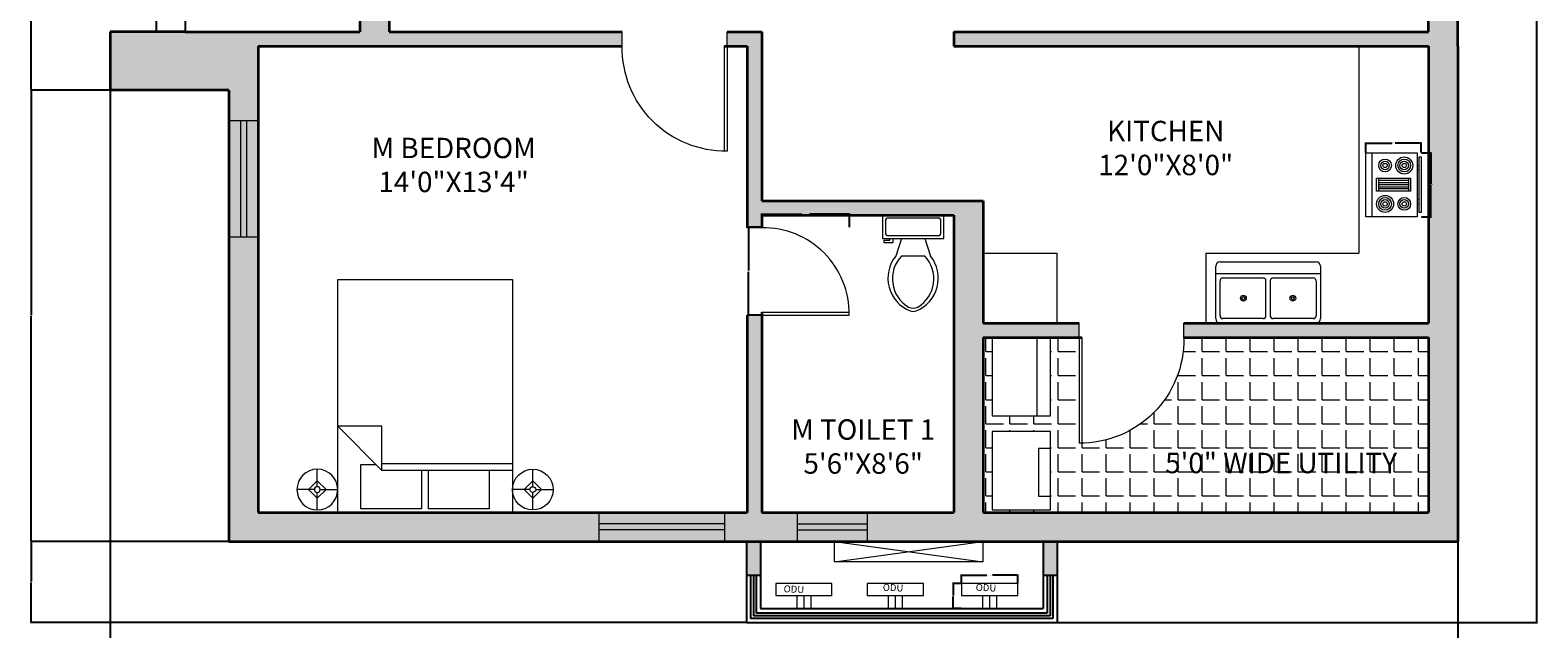
# Model space of a CAD drawing. Units: inches. Extents: x -382 to 250, y 518 to 1732.
# Tile 5 of 8: x -270 to 247, y 1167 to 1373. Entities that reach past the tile are written whole.
import ezdxf

# ---------------------------------------------------------------- set-up
doc = ezdxf.new("R2010")
doc.units = ezdxf.units.IN
doc.header["$MEASUREMENT"] = 0
for name, color, linetype, lineweight in [('A-ANNO-DIMS', 2, 'Continuous', 18), ('A-AREA-IDEN', 7, 'Continuous', 18), ('A-DOOR', 3, 'Continuous', 18), ('A-EQPM', 9, 'Continuous', 18), ('A-FLOR-CASE', 8, 'Continuous', 18), ('A-FLOR-EDGE', 7, 'Continuous', 25), ('A-FLOR-FIXT', 8, 'Continuous', 18), ('A-FLOR-PATT', 9, 'Continuous', 13), ('A-FLOR-SHFT', 8, 'Continuous', 18), ('A-FURN', 8, 'Continuous', 18), ('A-GLAZ', 4, 'Continuous', 18), ('A-WALL', 7, 'Continuous', 35), ('M-ANNO-TEXT', 7, 'Continuous', 13), ('M-HVAC-EQPM', 4, 'Continuous', 18)]:
    doc.layers.add(name, color=color, linetype=linetype, lineweight=lineweight)
doc.layers.add('A-GLAZ-PATT', color=143, linetype='Continuous', lineweight=13, true_color=0x7aafdf)
doc.layers.add('A-WALL-PATT', color=251, linetype='Continuous', lineweight=13, true_color=0x636466)
doc.styles.get("Standard").update_dxf_attribs({"font": 'arial.ttf'})
doc.dimstyles.get("Standard").update_dxf_attribs({"dimtxt": 0.18, "dimasz": 0.18, "dimexe": 0.18, "dimexo": 0.0625, "dimgap": 0.09, "dimtad": 0, "dimtih": 1, "dimtoh": 1, "dimdec": 4, "dimzin": 0, "dimdsep": 46, "dimtxsty": 'Standard', "dimcen": 0.09, "dimadec": 0, "dimazin": 0, "dimtfac": 1, "dimtdec": 4, "dimtofl": 0, "dimtmove": 0, "dimatfit": 3, "dimfxl": 1, "dimtolj": 1, "dimtzin": 0, "dimarcsym": 0})

# ---------------------------------------------------------------- blocks, each defined once
blk = doc.blocks.new('Bed - Queen')
for p, q in [((0, -80.00003), (0, 0)), ((0, 0), (59.99999, 0)), ((59.99999, 0), (59.99999, -80.00003)), ((7.99999, -1.2), (28.79998, -1.2)), ((7.99999, -14.4), (7.99999, -1.2)), ((28.79998, -1.2), (28.79998, -14.4)), ((31.19999, -1.2), (51.99999, -1.2)), ((31.19999, -14.4), (31.19999, -1.2)), ((51.99999, -1.2), (51.99999, -16.4)), ((0, -14.4), (44.8, -14.4)), ((59.99999, -29.6), (44.8, -14.4)), ((44.8, -14.4), (44.8, -29.6)), ((44.8, -16.8), (0, -16.8)), ((51.99999, -16.4), (46.79936, -16.4)), ((44.8, -29.6), (59.99999, -29.6)), ((59.99999, -80.00003), (0, -80.00003))]:
    blk.add_line(p, q)
blk = doc.blocks.new('Lamp - Table')
for p, q in [((0, 7), (0, 1)), ((-1, 0), (-7, 0)), ((0, 3), (-3, 0)), ((-3, 0), (0, -3)), ((3, 0), (0, 3)), ((0, -3), (3, 0)), ((1, 0), (7, 0)), ((0, -1), (0, -7))]:
    blk.add_line(p, q)
for radius in [7, 1]:
    blk.add_circle((0, 0), radius)
blk = doc.blocks.new('Range-Oven - 30 in top')
for p, q in [((0, -3), (30, -3)), ((12, -6), (18, -6)), ((13, -20), (13, -6)), ((14, -6), (14, -20)), ((15, -20), (15, -6)), ((16, -6), (16, -20)), ((17, -20), (17, -6)), ((18, -20), (12, -20)), ((6, -24), (6, -25)), ((8, -25), (8, -24)), ((22, -25), (22, -24)), ((24, -24), (24, -25))]:
    blk.add_line(p, q)
for points in [[(0, -24), (0, 0), (30, 0), (30, -24)], [(12, -21), (12, -5), (18, -5), (18, -21)], [(2, -26), (2, -25), (28, -25), (28, -26)]]:
    blk.add_lwpolyline(points, close=True)
for centre, radius in [((6, -9), 4), ((6, -9), 3), ((6, -9), 2), ((24, -9), 3), ((24, -9), 2), ((6, -9), 1), ((24, -18), 4), ((24, -9), 1), ((6, -18), 3), ((6, -18), 2), ((6, -18), 1), ((24, -18), 3), ((24, -18), 2), ((24, -18), 1)]:
    blk.add_circle(centre, radius)
blk = doc.blocks.new('Sink-double - 36 in top')
for p, q in [((-18, -4), (18, -4)), ((-0.75, -18.5), (-0.75, -6.5)), ((0.75, -6.5), (0.75, -18.5))]:
    blk.add_line(p, q)
for points in [[(-16.5, 0), (16.5, 0)], [(-18, -19.5), (-18, -1.5)], [(18, -1.5), (18, -19.5)], [(-16.5, -18.5), (-16.5, -6.5)], [(-15.5, -5.5), (-1.75, -5.5)], [(1.75, -5.5), (15.5, -5.5)], [(16.5, -6.5), (16.5, -18.5)], [(-1.75, -19.5), (-15.5, -19.5)], [(15.5, -19.5), (1.75, -19.5)], [(16.5, -21), (-16.5, -21)]]:
    blk.add_lwpolyline(points)
for centre, radius in [((-8.5, -12.5), 1), ((-8.5, -12.5), 0.5), ((8.5, -12.5), 1), ((8.5, -12.5), 0.5)]:
    blk.add_circle(centre, radius)
for centre, radius, start, end in [((-16.5, -1.5), 1.5, 90, 180), ((16.5, -1.5), 1.5, 0, 90), ((-15.5, -6.5), 1, 90, 180), ((-1.75, -6.5), 1, 0, 90), ((1.75, -6.5), 1, 90, 180), ((15.5, -6.5), 1, 0, 90), ((-16.5, -19.5), 1.5, 180, 270), ((-15.5, -18.5), 1, 180, 270), ((-1.75, -18.5), 1, 270, 0), ((1.75, -18.5), 1, 180, 270), ((15.5, -18.5), 1, 270, 0), ((16.5, -19.5), 1.5, 270, 0)]:
    blk.add_arc(centre, radius, start, end)
blk = doc.blocks.new('Toilet - top')
for p, q in [((9.5, -6), (9.5, -2)), ((-10, -8.5), (-8, -8.5)), ((-10, -9.5), (-10, -8.5)), ((-7, -9.5), (-10, -9.5)), ((-8, -8.5), (-8, -8)), ((-7, -8), (-7, -9.5)), ((-4, -8), (-6, -14)), ((4, -8), (6, -14)), ((4, -14), (-4, -14))]:
    blk.add_line(p, q)
blk.add_lwpolyline([(10.5, -8), (10.5, 0), (-10.5, 0), (-10.5, -8)], close=True)
for points in [[(-9.5, -2), (-9.5, -6)], [(8.5, -1), (-8.5, -1)], [(-8.5, -7), (8.5, -7)]]:
    blk.add_lwpolyline(points)
for centre, radius, start, end in [((-8.62, -1.88), 0.884, 81.8699, 188.1301), ((8.62, -1.88), 0.884, 351.8699, 98.1301), ((-8.62, -6.12), 0.884, 171.8699, 278.1301), ((8.62, -6.12), 0.884, 261.8699, 8.1301), ((3.52, -21.58), 12.17, 141.4691, 247.9714), ((4.2, -21.82), 11.33, 136.3677, 238.9468), ((-3.52, -21.58), 12.17, 292.0284, 38.5307), ((-4.2, -21.82), 11.33, 301.053, 43.6321), ((0, -27.88), 4, 245.7318, 294.2682), ((0, -29), 4, 254.8605, 285.1395)]:
    blk.add_arc(centre, radius, start, end)
blk = doc.blocks.new('WIN-43_2IN')
for p, q in [((0, 10), (0, 0)), ((0, 6), (43.2, 6)), ((43.2, 10), (43.2, 0)), ((0, 4), (43.2, 4))]:
    blk.add_line(p, q)
blk = doc.blocks.new('WIN-40IN')
for p, q in [((10, 40), (0, 40)), ((4, 40), (4, 0)), ((6, 40), (6, 0)), ((10, 0), (0, 0))]:
    blk.add_line(p, q)
blk = doc.blocks.new('WIN-24IN')
for p, q in [((0, 0), (0, 10)), ((0, 6), (24, 6)), ((24, 0), (24, 10)), ((0, 4), (24, 4))]:
    blk.add_line(p, q)
blk = doc.blocks.new('DOOR-SWING-36IN')
for p, q in [((-1, 0), (-1, 36)), ((0, 0), (0, 36))]:
    blk.add_line(p, q)
blk.add_arc((-0.5, 0.5), 35.5, 89.1931, 180.8069)
blk = doc.blocks.new('DOOR-SWING-30IN')
for p, q in [((0, 1), (30, 1)), ((0, 0), (30, 0))]:
    blk.add_line(p, q)
blk.add_arc((0.5, 0.5), 29.5, 359.029, 90.971)
blk = doc.blocks.new('ODU-LEDGE-SMALL')
for p, q in [((7.26, 4.51), (7.26, 0)), ((9.66, 4.51), (9.66, 0)), ((12.06, 4.51), (12.06, 0))]:
    blk.add_line(p, q)
blk.add_lwpolyline([(0, 4.51), (19.32, 4.51), (19.32, 8.62), (0, 8.62)], close=True)
blk = doc.blocks.new('DOOR-SWING-36IN-OFFSET')
for p, q in [((0, 0), (0, 36)), ((1, -0.22), (1, 36))]:
    blk.add_line(p, q)
blk.add_arc((0.5, 0.5), 35.5, 359.1931, 90.8069)
blk = doc.blocks.new('*D48')
at = {"layer": 'A-ANNO-DIMS', "color": 0, "lineweight": -2, "transparency": 16777216}
for p, q in [((207.33, 1330.55), (210.75, 1330.55)), ((210.57, 1330.37), (210.57, 1319.75)), ((210.57, 1308.76), (210.57, 1319.38)), ((207.33, 1308.58), (210.75, 1308.58))]:
    blk.add_line(p, q, dxfattribs=at)
at = {"layer": 'A-ANNO-DIMS', "color": 0, "transparency": 16777216}
for points in [[(210.54, 1330.37), (210.6, 1330.37), (210.57, 1330.55)], [(210.54, 1308.76), (210.6, 1308.76), (210.57, 1308.58)]]:
    blk.add_solid(points, dxfattribs=at)
at = {"layer": 'Defpoints', "color": 0, "transparency": 16777216}
for p in [(207.27, 1330.55), (210.57, 1330.55), (207.27, 1308.58)]:
    blk.add_point(p, dxfattribs=at)
at = {"layer": 'A-ANNO-DIMS', "color": 0, "transparency": 16777216, "insert": (210.57, 1319.57), "char_height": 0.18, "attachment_point": 5}
blk.add_mtext('\\A1;RANGE 22 TYP.', dxfattribs=at)
blk = doc.blocks.new('*D49')
at = {"layer": 'A-ANNO-DIMS', "color": 0, "lineweight": -2, "transparency": 16777216}
for p, q in [((188.23, 1330.61), (188.23, 1334.03)), ((188.41, 1333.85), (197.23, 1333.85)), ((207.09, 1333.85), (198.27, 1333.85)), ((207.27, 1330.61), (207.27, 1334.03))]:
    blk.add_line(p, q, dxfattribs=at)
at = {"layer": 'A-ANNO-DIMS', "color": 0, "transparency": 16777216}
for points in [[(188.41, 1333.88), (188.41, 1333.82), (188.23, 1333.85)], [(207.09, 1333.88), (207.09, 1333.82), (207.27, 1333.85)]]:
    blk.add_solid(points, dxfattribs=at)
at = {"layer": 'Defpoints', "color": 0, "transparency": 16777216}
for p in [(188.23, 1333.85), (188.23, 1330.55), (207.27, 1330.55)]:
    blk.add_point(p, dxfattribs=at)
at = {"layer": 'A-ANNO-DIMS', "color": 0, "transparency": 16777216, "insert": (197.75, 1333.85), "char_height": 0.18, "attachment_point": 5}
blk.add_mtext('\\A1;19 TYP.', dxfattribs=at)
blk = doc.blocks.new('*D54')
at = {"layer": 'A-ANNO-DIMS', "color": 0, "lineweight": -2, "transparency": 16777216}
for p, q in [((49.35, 1182.69), (49.35, 1185.7)), ((49.53, 1185.52), (58.04, 1185.52)), ((68.49, 1185.52), (59.97, 1185.52)), ((68.67, 1182.69), (68.67, 1185.7))]:
    blk.add_line(p, q, dxfattribs=at)
at = {"layer": 'A-ANNO-DIMS', "color": 0, "transparency": 16777216}
for points in [[(49.53, 1185.55), (49.53, 1185.49), (49.35, 1185.52)], [(68.49, 1185.55), (68.49, 1185.49), (68.67, 1185.52)]]:
    blk.add_solid(points, dxfattribs=at)
at = {"layer": 'Defpoints', "color": 0, "transparency": 16777216}
for p in [(49.35, 1182.62), (68.67, 1185.52), (68.67, 1182.62)]:
    blk.add_point(p, dxfattribs=at)
at = {"layer": 'A-ANNO-DIMS', "color": 0, "transparency": 16777216, "insert": (59.01, 1185.52), "char_height": 0.18, "attachment_point": 5}
blk.add_mtext('\\A1;ODU-S 19 TYP.', dxfattribs=at)
blk = doc.blocks.new('*D55')
at = {"layer": 'A-ANNO-DIMS', "color": 0, "lineweight": -2, "transparency": 16777216}
for p, q in [((49.28, 1182.62), (46.27, 1182.62)), ((46.45, 1182.44), (46.45, 1178.5)), ((46.45, 1174.18), (46.45, 1178.13)), ((49.28, 1174), (46.27, 1174))]:
    blk.add_line(p, q, dxfattribs=at)
at = {"layer": 'A-ANNO-DIMS', "color": 0, "transparency": 16777216}
for points in [[(46.42, 1182.44), (46.48, 1182.44), (46.45, 1182.62)], [(46.42, 1174.18), (46.48, 1174.18), (46.45, 1174)]]:
    blk.add_solid(points, dxfattribs=at)
at = {"layer": 'Defpoints', "color": 0, "transparency": 16777216}
for p in [(46.45, 1182.62), (49.35, 1182.62), (49.35, 1174)]:
    blk.add_point(p, dxfattribs=at)
at = {"layer": 'A-ANNO-DIMS', "color": 0, "transparency": 16777216, "insert": (46.45, 1178.31), "char_height": 0.18, "attachment_point": 5}
blk.add_mtext('\\A1;9 TYP.', dxfattribs=at)
blk = doc.blocks.new('*D64')
at = {"layer": 'A-ANNO-DIMS', "color": 0, "lineweight": -2, "transparency": 16777216}
for p, q in [((-19.22, 1305), (-19.22, 1309.63)), ((-19.04, 1309.45), (-5.45, 1309.45)), ((10.74, 1309.45), (-2.84, 1309.45)), ((10.92, 1305), (10.92, 1309.63))]:
    blk.add_line(p, q, dxfattribs=at)
at = {"layer": 'A-ANNO-DIMS', "color": 0, "transparency": 16777216}
for points in [[(-19.04, 1309.48), (-19.04, 1309.42), (-19.22, 1309.45)], [(10.74, 1309.48), (10.74, 1309.42), (10.92, 1309.45)]]:
    blk.add_solid(points, dxfattribs=at)
at = {"layer": 'Defpoints', "color": 0, "transparency": 16777216}
for p in [(-19.22, 1304.93), (10.92, 1309.45), (10.92, 1304.93)]:
    blk.add_point(p, dxfattribs=at)
at = {"layer": 'A-ANNO-DIMS', "color": 0, "transparency": 16777216, "insert": (-4.15, 1309.45), "char_height": 0.18, "attachment_point": 5}
blk.add_mtext('\\A1;BATH DOOR 30 TYP.', dxfattribs=at)
blk = doc.blocks.new('*D65')
at = {"layer": 'A-ANNO-DIMS', "color": 0, "lineweight": -2, "transparency": 16777216}
for p, q in [((-19.28, 1304.93), (-23.92, 1304.93)), ((-23.74, 1304.75), (-23.74, 1290.05)), ((-23.74, 1274.98), (-23.74, 1289.68)), ((-19.28, 1274.8), (-23.92, 1274.8))]:
    blk.add_line(p, q, dxfattribs=at)
at = {"layer": 'A-ANNO-DIMS', "color": 0, "transparency": 16777216}
for points in [[(-23.77, 1304.75), (-23.71, 1304.75), (-23.74, 1304.93)], [(-23.77, 1274.98), (-23.71, 1274.98), (-23.74, 1274.8)]]:
    blk.add_solid(points, dxfattribs=at)
at = {"layer": 'Defpoints', "color": 0, "transparency": 16777216}
for p in [(-23.74, 1304.93), (-19.22, 1304.93), (-19.22, 1274.8)]:
    blk.add_point(p, dxfattribs=at)
at = {"layer": 'A-ANNO-DIMS', "color": 0, "transparency": 16777216, "insert": (-23.74, 1289.86), "char_height": 0.18, "attachment_point": 5}
blk.add_mtext('\\A1;30 TYP.', dxfattribs=at)
blk = doc.blocks.new('*D86')
at = {"layer": 'A-ANNO-DIMS', "color": 0, "lineweight": -2, "transparency": 16777216}
for p, q in [((-242.98, 1352.01), (-242.98, 1141.82)), ((219.78, 1197.01), (219.78, 1141.82)), ((-242.8, 1142), (-11.99, 1142)), ((219.6, 1142), (-11.2, 1142))]:
    blk.add_line(p, q, dxfattribs=at)
at = {"layer": 'A-ANNO-DIMS', "color": 0, "transparency": 16777216}
for points in [[(-242.8, 1142.03), (-242.8, 1141.97), (-242.98, 1142)], [(219.6, 1142.03), (219.6, 1141.97), (219.78, 1142)]]:
    blk.add_solid(points, dxfattribs=at)
at = {"layer": 'Defpoints', "color": 0, "transparency": 16777216}
for p in [(-242.98, 1352.07), (219.78, 1197.07), (219.78, 1142)]:
    blk.add_point(p, dxfattribs=at)
at = {"layer": 'A-ANNO-DIMS', "color": 0, "transparency": 16777216, "insert": (-11.6, 1142), "char_height": 0.18, "attachment_point": 5}
blk.add_mtext('\\A1;462.8', dxfattribs=at)
blk = doc.blocks.new('*D87')
at = {"layer": 'A-ANNO-DIMS', "color": 0, "lineweight": -2, "transparency": 16777216}
for p, q in [((87.85, 1704.87), (247.16, 1704.87)), ((246.98, 1704.69), (246.98, 1437.22)), ((246.98, 1169.38), (246.98, 1436.85)), ((82.25, 1169.2), (247.16, 1169.2))]:
    blk.add_line(p, q, dxfattribs=at)
at = {"layer": 'A-ANNO-DIMS', "color": 0, "transparency": 16777216}
for points in [[(246.95, 1704.69), (247.01, 1704.69), (246.98, 1704.87)], [(246.95, 1169.38), (247.01, 1169.38), (246.98, 1169.2)]]:
    blk.add_solid(points, dxfattribs=at)
at = {"layer": 'Defpoints', "color": 0, "transparency": 16777216}
for p in [(87.78, 1704.87), (246.98, 1704.87), (82.19, 1169.2)]:
    blk.add_point(p, dxfattribs=at)
at = {"layer": 'A-ANNO-DIMS', "color": 0, "transparency": 16777216, "insert": (246.98, 1437.03), "char_height": 0.18, "attachment_point": 5}
blk.add_mtext('\\A1;535.7', dxfattribs=at)
blk = doc.blocks.new('*D91')
at = {"layer": 'A-ANNO-DIMS', "color": 0, "lineweight": -2, "transparency": 16777216}
for p, q in [((-202.28, 1352.07), (-270.36, 1352.07)), ((-270.18, 1351.89), (-270.18, 1274.75)), ((-270.18, 1197.25), (-270.18, 1274.39)), ((-202.28, 1197.07), (-270.36, 1197.07))]:
    blk.add_line(p, q, dxfattribs=at)
at = {"layer": 'A-ANNO-DIMS', "color": 0, "transparency": 16777216}
for points in [[(-270.21, 1351.89), (-270.15, 1351.89), (-270.18, 1352.07)], [(-270.21, 1197.25), (-270.15, 1197.25), (-270.18, 1197.07)]]:
    blk.add_solid(points, dxfattribs=at)
at = {"layer": 'Defpoints', "color": 0, "transparency": 16777216}
for p in [(-270.18, 1352.07), (-202.22, 1352.07), (-202.22, 1197.07)]:
    blk.add_point(p, dxfattribs=at)
at = {"layer": 'A-ANNO-DIMS', "color": 0, "transparency": 16777216, "insert": (-270.18, 1274.57), "char_height": 0.18, "attachment_point": 5}
blk.add_mtext('\\A1;155', dxfattribs=at)
blk = doc.blocks.new('*D92')
at = {"layer": 'A-ANNO-DIMS', "color": 0, "lineweight": -2, "transparency": 16777216}
for p, q in [((-202.28, 1504.07), (-270.36, 1504.07)), ((-270.18, 1503.89), (-270.18, 1428.25)), ((-270.18, 1352.25), (-270.18, 1427.89)), ((-243.04, 1352.07), (-270.36, 1352.07))]:
    blk.add_line(p, q, dxfattribs=at)
at = {"layer": 'A-ANNO-DIMS', "color": 0, "transparency": 16777216}
for points in [[(-270.21, 1503.89), (-270.15, 1503.89), (-270.18, 1504.07)], [(-270.21, 1352.25), (-270.15, 1352.25), (-270.18, 1352.07)]]:
    blk.add_solid(points, dxfattribs=at)
at = {"layer": 'Defpoints', "color": 0, "transparency": 16777216}
for p in [(-270.18, 1504.07), (-202.22, 1504.07), (-242.98, 1352.07)]:
    blk.add_point(p, dxfattribs=at)
at = {"layer": 'A-ANNO-DIMS', "color": 0, "transparency": 16777216, "insert": (-270.18, 1428.07), "char_height": 0.18, "attachment_point": 5}
blk.add_mtext('\\A1;152', dxfattribs=at)
blk = doc.blocks.new('*D94')
at = {"layer": 'A-ANNO-DIMS', "color": 0, "lineweight": -2, "transparency": 16777216}
for p, q in [((-202.28, 1197.07), (-270.36, 1197.07)), ((-270.18, 1196.89), (-270.18, 1183.32)), ((-270.18, 1169.38), (-270.18, 1182.95)), ((-24.55, 1169.2), (-270.36, 1169.2))]:
    blk.add_line(p, q, dxfattribs=at)
at = {"layer": 'A-ANNO-DIMS', "color": 0, "transparency": 16777216}
for points in [[(-270.21, 1196.89), (-270.15, 1196.89), (-270.18, 1197.07)], [(-270.21, 1169.38), (-270.15, 1169.38), (-270.18, 1169.2)]]:
    blk.add_solid(points, dxfattribs=at)
at = {"layer": 'Defpoints', "color": 0, "transparency": 16777216}
for p in [(-270.18, 1197.07), (-202.22, 1197.07), (-24.49, 1169.2)]:
    blk.add_point(p, dxfattribs=at)
at = {"layer": 'A-ANNO-DIMS', "color": 0, "transparency": 16777216, "insert": (-270.18, 1183.13), "char_height": 0.18, "attachment_point": 5}
blk.add_mtext('\\A1;27.87', dxfattribs=at)

msp = doc.modelspace()

# ---------------------------------------------------------------- hatches: boundary and pattern name
at = {"layer": 'A-FLOR-PATT'}
h = msp.add_hatch(dxfattribs=at)
h.set_pattern_fill('ANGLE', color=256, scale=30)
h.set_pattern_definition([(0, (0, 0), (0, 8.25), [6, -2.25]), (90, (0, 0), (-8.25, 5e-16), [6, -2.25])])
h.paths.add_polyline_path([(209.785, 1267.0687), (125.7302, 1267.0687), (125.7302, 1266.8519, -0.4224878), (89.7302, 1230.8519), (89.7302, 1267.0687), (79.9772, 1267.0687), (79.9772, 1240.2287), (75.2198, 1240.2287), (59.9383, 1240.2287), (59.9383, 1267.0687), (56.785, 1267.0687), (56.785, 1207.0687), (209.785, 1207.0687)])
h.paths.add_polyline_path([(79.9772, 1234.8286), (79.9772, 1207.9886), (59.9383, 1207.9886), (59.9383, 1234.8286)], flags=16)
h.paths.add_polyline_path([(79.9772, 1228.9541), (79.9772, 1212.6048), (75.8027, 1212.6048), (75.8027, 1228.9541)], flags=0)
h.paths.add_polyline_path([(115.4168, 1216.6676), (202.5014, 1216.6676), (202.5014, 1231.0925), (115.4168, 1231.0925)], flags=24)
at = {"layer": 'A-GLAZ-PATT'}
h = msp.add_hatch(color=256, dxfattribs=at)
h.dxf.hatch_style = 1
h.paths.add_polyline_path([(-198.215, 1341.5341), (-202.215, 1341.5341), (-202.215, 1301.5341), (-198.215, 1301.5341)])
h = msp.add_hatch(color=256, dxfattribs=at)
h.dxf.hatch_style = 1
h.paths.add_polyline_path([(-196.215, 1341.5341), (-198.215, 1341.5341), (-198.215, 1301.5341), (-196.215, 1301.5341)])
h = msp.add_hatch(color=256, dxfattribs=at)
h.dxf.hatch_style = 1
h.paths.add_polyline_path([(-192.215, 1341.5341), (-196.215, 1341.5341), (-196.215, 1301.5341), (-192.215, 1301.5341)])
h = msp.add_hatch(color=256, dxfattribs=at)
h.dxf.hatch_style = 1
h.paths.add_polyline_path([(-31.9223, 1207.0687), (-75.1223, 1207.0687), (-75.1223, 1203.0687), (-31.9223, 1203.0687)])
h = msp.add_hatch(color=256, dxfattribs=at)
h.dxf.hatch_style = 1
h.paths.add_polyline_path([(17.0948, 1207.0687), (-6.9052, 1207.0687), (-6.9052, 1203.0687), (17.0948, 1203.0687)])
h = msp.add_hatch(color=256, dxfattribs=at)
h.dxf.hatch_style = 1
h.paths.add_polyline_path([(-31.9223, 1203.0687), (-75.1223, 1203.0687), (-75.1223, 1201.0687), (-31.9223, 1201.0687)])
h = msp.add_hatch(color=256, dxfattribs=at)
h.dxf.hatch_style = 1
h.paths.add_polyline_path([(17.0948, 1203.0687), (-6.9052, 1203.0687), (-6.9052, 1201.0687), (17.0948, 1201.0687)])
h = msp.add_hatch(color=256, dxfattribs=at)
h.dxf.hatch_style = 1
h.paths.add_polyline_path([(-31.9223, 1201.0687), (-75.1223, 1201.0687), (-75.1223, 1197.0687), (-31.9223, 1197.0687)])
h = msp.add_hatch(color=256, dxfattribs=at)
h.dxf.hatch_style = 1
h.paths.add_polyline_path([(17.0948, 1201.0687), (-6.9052, 1201.0687), (-6.9052, 1197.0687), (17.0948, 1197.0687)])
at = {"layer": 'A-WALL-PATT'}
h = msp.add_hatch(color=256, dxfattribs=at)
h.dxf.hatch_style = 1
h.paths.add_polyline_path([(219.785, 1367.0687), (219.785, 1447.835), (209.785, 1447.835), (209.785, 1372.0687), (46.785, 1372.0687), (46.785, 1367.0687), (209.785, 1367.0687), (209.785, 1272.0687), (125.7302, 1272.0687), (125.7302, 1267.0687), (209.785, 1267.0687), (209.785, 1207.0687), (56.785, 1207.0687), (56.785, 1267.0687), (89.7302, 1267.0687), (89.7302, 1272.0687), (56.785, 1272.0687), (56.785, 1314.0687), (-19.215, 1314.0687), (-19.215, 1372.0687), (-31.1575, 1372.0687), (-31.1575, 1367.0687), (-24.215, 1367.0687), (-24.215, 1304.7972), (-19.215, 1304.7972), (-19.215, 1309.0687), (46.785, 1309.0687), (46.785, 1207.0687), (17.0948, 1207.0687), (17.0948, 1197.0687), (56.7186, 1197.0687), (219.785, 1197.0687)])
h = msp.add_hatch(color=256, dxfattribs=at)
h.dxf.hatch_style = 1
h.paths.add_polyline_path([(-147.215, 1390.0687), (-157.215, 1390.0687), (-157.215, 1372.0687), (-217.215, 1372.0687), (-242.9787, 1372.0687), (-242.9787, 1352.0687), (-202.215, 1352.0687), (-202.215, 1341.5341), (-192.215, 1341.5341), (-192.215, 1367.0687), (-67.1575, 1367.0687), (-67.1575, 1372.0687), (-147.215, 1372.0687)])
h = msp.add_hatch(color=256, dxfattribs=at)
h.dxf.hatch_style = 1
h.paths.add_polyline_path([(-75.1223, 1207.0687), (-192.215, 1207.0687), (-192.215, 1301.5341), (-202.215, 1301.5341), (-202.215, 1197.0687), (-75.1223, 1197.0687)])
h = msp.add_hatch(color=256, dxfattribs=at)
h.dxf.hatch_style = 1
h.paths.add_polyline_path([(-6.9052, 1207.0687), (-19.215, 1207.0687), (-19.215, 1274.7972), (-24.215, 1274.7972), (-24.215, 1207.0687), (-31.9223, 1207.0687), (-31.9223, 1197.0687), (-6.9052, 1197.0687)])
h = msp.add_hatch(color=256, dxfattribs=at)
h.dxf.hatch_style = 1
h.paths.add_polyline_path([(-19.6862, 1197.0687), (-24.4916, 1197.0687), (-24.4916, 1185.4874), (-19.6862, 1185.4874)], flags=17)
h = msp.add_hatch(color=256, dxfattribs=at)
h.dxf.hatch_style = 1
h.paths.add_polyline_path([(82.1869, 1197.0687), (77.3816, 1197.0687), (77.3816, 1185.5359), (82.1869, 1185.5359)])

# ---------------------------------------------------------------- linework, layer by layer
at = {"layer": 'A-DOOR'}
for p, q in [((-67.1575, 1367.0687), (-67.1575, 1372.0687)), ((-31.1575, 1367.0687), (-31.1575, 1372.0687)), ((-19.215, 1304.7972), (-24.215, 1304.7972)), ((-19.215, 1274.7972), (-24.215, 1274.7972)), ((89.7302, 1266.8519), (89.7302, 1272.0687)), ((125.7302, 1266.8519), (125.7302, 1272.0687))]:
    msp.add_line(p, q, dxfattribs=at)
at = {"layer": 'A-EQPM'}
for points in [[(59.9383, 1240.2287), (79.9772, 1240.2287), (79.9772, 1267.0687), (59.9383, 1267.0687)], [(79.9772, 1267.0687), (75.2198, 1267.0687), (75.2198, 1240.2287), (79.9772, 1240.2287)], [(59.9383, 1207.9886), (79.9772, 1207.9886), (79.9772, 1234.8286), (59.9383, 1234.8286)], [(79.9772, 1228.9541), (75.8027, 1228.9541), (75.8027, 1212.6048), (79.9772, 1212.6048)]]:
    msp.add_lwpolyline(points, close=True, dxfattribs=at)
at = {"layer": 'A-FLOR-CASE'}
for p, q in [((185.785, 1367.0687), (185.785, 1296.0687)), ((56.785, 1296.0687), (82.0525, 1296.0687)), ((82.0525, 1296.0687), (82.0525, 1272.0687)), ((133.285, 1296.0687), (133.285, 1272.0687)), ((133.285, 1296.0687), (185.785, 1296.0687))]:
    msp.add_line(p, q, dxfattribs=at)
at = {"layer": 'A-FLOR-EDGE'}
for p, q in [((-227.215, 1492.0687), (-227.215, 1372.0687)), ((-217.215, 1492.0687), (-217.215, 1372.0687)), ((-24.4916, 1197.0687), (-24.4916, 1169.1977)), ((-19.6862, 1197.0687), (-19.6862, 1174.0031)), ((77.3816, 1197.0687), (77.3816, 1174.0031)), ((82.1869, 1197.0687), (82.1869, 1169.1977)), ((-24.4916, 1185.4874), (-19.6862, 1185.4874)), ((-23.05, 1185.5359), (-23.05, 1170.584)), ((-22.0889, 1185.5359), (-22.0889, 1171.545)), ((-21.1278, 1185.5359), (-21.1278, 1172.5061)), ((77.3816, 1185.5359), (82.1869, 1185.5359)), ((78.8232, 1185.5359), (78.8232, 1172.5061)), ((79.7843, 1185.5359), (79.7843, 1171.545)), ((80.7453, 1185.5359), (80.7453, 1170.584)), ((80.7453, 1170.584), (-23.05, 1170.584)), ((79.7843, 1171.545), (-22.0889, 1171.545)), ((78.8232, 1172.5061), (-21.1278, 1172.5061)), ((-19.6862, 1174.0031), (77.3816, 1174.0031)), ((-24.4916, 1169.1977), (82.1869, 1169.1977))]:
    msp.add_line(p, q, dxfattribs=at)
at = {"layer": 'A-FLOR-SHFT'}
for p, q in [((5.7821, 1197.0687), (56.7186, 1190.1249)), ((5.7821, 1190.1249), (56.7186, 1197.0687))]:
    msp.add_line(p, q, dxfattribs=at)
msp.add_lwpolyline([(5.7821, 1197.0687), (56.7186, 1197.0687), (56.7186, 1190.1249), (5.7821, 1190.1249)], close=True, dxfattribs=at)
at = {"layer": 'A-WALL'}
for p, q in [((-157.215, 1504.0687), (-157.215, 1372.0687)), ((-147.215, 1504.0687), (-147.215, 1372.0687)), ((209.785, 1372.0687), (209.785, 1447.835)), ((219.785, 1367.0687), (219.785, 1447.835)), ((-217.215, 1372.0687), (-242.9787, 1372.0687)), ((-242.9787, 1372.0687), (-242.9787, 1352.0687)), ((-217.215, 1372.0687), (-157.215, 1372.0687)), ((-192.215, 1367.0687), (-67.1575, 1367.0687)), ((-192.215, 1367.0687), (-192.215, 1207.0687)), ((-147.215, 1372.0687), (-67.1575, 1372.0687)), ((-32.1575, 1367.0687), (-24.215, 1367.0687)), ((-31.1575, 1372.0687), (-19.215, 1372.0687)), ((-24.215, 1367.0687), (-24.215, 1304.7972)), ((-19.215, 1372.0687), (-19.215, 1314.0687)), ((46.785, 1372.0687), (46.785, 1367.0687)), ((46.785, 1372.0687), (209.785, 1372.0687)), ((46.785, 1367.0687), (209.785, 1367.0687)), ((209.785, 1367.0687), (209.785, 1272.0687)), ((219.785, 1367.0687), (219.785, 1197.0687)), ((-202.215, 1352.0687), (-242.9787, 1352.0687)), ((-202.215, 1352.0687), (-202.215, 1197.0687)), ((-19.215, 1314.0687), (56.785, 1314.0687)), ((56.785, 1314.0687), (56.785, 1272.0687)), ((-19.215, 1309.0687), (46.785, 1309.0687)), ((-19.215, 1309.0687), (-19.215, 1304.7972)), ((46.785, 1309.0687), (46.785, 1207.0687)), ((-24.215, 1274.7972), (-24.215, 1207.0687)), ((-19.215, 1275.7972), (-19.215, 1207.0687)), ((56.785, 1272.0687), (89.7302, 1272.0687)), ((125.7302, 1272.0687), (209.785, 1272.0687)), ((56.785, 1267.0687), (90.7302, 1267.0687)), ((56.785, 1267.0687), (56.785, 1207.0687)), ((125.7302, 1267.0687), (209.785, 1267.0687)), ((209.785, 1267.0687), (209.785, 1207.0687)), ((-192.215, 1207.0687), (-24.215, 1207.0687)), ((-19.215, 1207.0687), (46.785, 1207.0687)), ((56.785, 1207.0687), (209.785, 1207.0687)), ((-202.215, 1197.0687), (219.785, 1197.0687))]:
    msp.add_line(p, q, dxfattribs=at)
at = {"layer": 'M-HVAC-EQPM'}
msp.add_lwpolyline([(16.9551, 1178.5097), (36.2761, 1178.5097), (36.2761, 1182.6247), (16.9551, 1182.6247)], close=True, dxfattribs=at)

# ---------------------------------------------------------------- block references
at = {"layer": 'A-DOOR', "extrusion": (0, 0, -1), "zscale": -1, "rotation": 180}
for name, p in [('DOOR-SWING-36IN', (31.1575, 1367.0687)), ('DOOR-SWING-36IN-OFFSET', (-89.7302, 1266.8519))]:
    msp.add_blockref(name, p, dxfattribs=at)
at = {"layer": 'A-DOOR'}
msp.add_blockref('DOOR-SWING-30IN', (-19.215, 1274.7972), dxfattribs=at)
at = {"layer": 'A-EQPM', "xscale": 0.7322775252250638, "yscale": 0.7322775252250638, "zscale": 0.7322775252250638, "rotation": 90}
msp.add_blockref('Range-Oven - 30 in top', (188.2321, 1308.5819), dxfattribs=at)
at = {"layer": 'A-FLOR-FIXT'}
for name, p in [('Toilet - top', (32.7533, 1309.0687)), ('Sink-double - 36 in top', (154.6547, 1293.0687))]:
    msp.add_blockref(name, p, dxfattribs=at)
at = {"layer": 'A-FURN', "rotation": 180}
for name, p in [('Bed - Queen', (-104.8707, 1207.0687)), ('Lamp - Table', (-97.8707, 1214.8801))]:
    msp.add_blockref(name, p, dxfattribs=at)
at = {"layer": 'A-FURN', "xscale": -1, "rotation": 180}
msp.add_blockref('Lamp - Table', (-171.8707, 1214.8801), dxfattribs=at)
at = {"layer": 'A-GLAZ'}
for name, p in [('WIN-40IN', (-202.215, 1301.5337)), ('WIN-24IN', (-6.9048, 1197.069))]:
    msp.add_blockref(name, p, dxfattribs=at)
at = {"layer": 'A-GLAZ', "rotation": 180}
msp.add_blockref('WIN-43_2IN', (-31.9223, 1207.0684), dxfattribs=at)
at = {"layer": 'M-HVAC-EQPM'}
for p in [(-14.442, 1174.003), (16.9546, 1174.003), (49.3456, 1174.003)]:
    msp.add_blockref('ODU-LEDGE-SMALL', p, dxfattribs=at)

# ---------------------------------------------------------------- texts
at = {"layer": 'A-AREA-IDEN', "char_height": 7, "attachment_point": 1}
for s, width, insert in [('\\pxqc;KITCHEN\\P12\'0"X8\'0"', 79.656175, (79.6751, 1341.4996)), ('\\pxqc;M BEDROOM \\P14\'0"X13\'4"', 79.656175, (-164.8707, 1335.6712)), ('\\pxqc;M TOILET 1\\P5\'6"X8\'6"', 79.656175, (-24.215, 1239.0027)), ('\\pxqc;\\P5\'0" WIDE UTILITY', 101.975496, (108.136, 1239.1852))]:
    msp.add_mtext_dynamic_manual_height_columns(s, width=width, gutter_width=1, heights=[0], dxfattribs=dict(at, insert=insert))
at = {"layer": 'M-ANNO-TEXT', "char_height": 2.40267, "attachment_point": 7, "rotation": 357.66503}
for insert in [(-11.7695, 1179.6366), (22.2968, 1180.1405), (54.2096, 1180.1405)]:
    msp.add_mtext_dynamic_manual_height_columns('ODU', width=6.558487, gutter_width=0.4805, heights=[0], dxfattribs=dict(at, insert=insert))

# ---------------------------------------------------------------- dimensions: what is measured, and where the dimension line sits
at = {"layer": 'A-ANNO-DIMS'}
for base, p1, p2, override, picture, middle in [((246.985, 1704.8705), (82.1869, 1169.1977), (87.785, 1704.8705), {"dimdec": 1, "dimlfac": 1, "dimrnd": 0, "dimzin": 0, "dimdsep": 46, "dimlunit": 2}, '*D87', (246.985, 1437.0341)), ((-270.1787, 1504.0687), (-242.9787, 1352.0687), (-202.215, 1504.0687), {"dimdec": 0, "dimlfac": 1, "dimrnd": 0, "dimzin": 0, "dimdsep": 46, "dimlunit": 2}, '*D92', (-270.1787, 1428.0687)), ((-270.1787, 1352.0687), (-202.215, 1197.0687), (-202.215, 1352.0687), {"dimdec": 0, "dimlfac": 1, "dimrnd": 0, "dimzin": 0, "dimdsep": 46, "dimlunit": 2}, '*D91', (-270.1787, 1274.5687)), ((-270.1787, 1197.0687), (-24.4916, 1169.1977), (-202.215, 1197.0687), {"dimdec": 2, "dimlfac": 1, "dimrnd": 0, "dimzin": 0, "dimdsep": 46, "dimlunit": 2}, '*D94', (-270.1787, 1183.1332))]:
    dim = msp.add_linear_dim(base=base, p1=p1, p2=p2, angle=90, dimstyle='Standard', override=override, dxfattribs=at)
    dim.commit()
    dim.dimension.update_dxf_attribs({"geometry": picture, "text_midpoint": middle})
dim = msp.add_linear_dim(base=(219.785, 1141.9977), p1=(-242.9787, 1352.0687), p2=(219.785, 1197.0687), dimstyle='Standard', override={"dimdec": 1, "dimlfac": 1, "dimrnd": 0, "dimzin": 0, "dimdsep": 46, "dimlunit": 2}, dxfattribs=at)
dim.commit()
dim.dimension.update_dxf_attribs({"geometry": '*D86', "text_midpoint": (-11.5969, 1141.9977)})
for base, p1, p2, angle, text, picture, middle in [((188.2321, 1333.8454), (207.2713, 1330.5502), (188.2321, 1330.5502), 180, '<> TYP.', '*D49', (197.7517, 1333.8454)), ((210.5665, 1330.5502), (207.2713, 1308.5819), (207.2713, 1330.5502), 90, 'RANGE <> TYP.', '*D48', (210.5665, 1319.566)), ((-23.7354, 1304.9327), (-19.215, 1274.7972), (-19.215, 1304.9327), 90, '<> TYP.', '*D65', (-23.7354, 1289.8649)), ((46.448, 1182.6247), (49.3461, 1174.0031), (49.3461, 1182.6247), 90, '<> TYP.', '*D55', (46.448, 1178.3139))]:
    dim = msp.add_linear_dim(base=base, p1=p1, p2=p2, angle=angle, text=text, dimstyle='Standard', override={"dimdec": 0, "dimlfac": 1, "dimrnd": 0, "dimzin": 0, "dimdsep": 46, "dimlunit": 2}, dxfattribs=at)
    dim.commit()
    dim.dimension.update_dxf_attribs({"geometry": picture, "text_midpoint": middle})
for base, p1, p2, text, picture, middle in [((10.9205, 1309.453), (-19.215, 1304.9327), (10.9205, 1304.9327), 'BATH DOOR <> TYP.', '*D64', (-4.1473, 1309.453)), ((68.6671, 1185.5228), (49.3461, 1182.6247), (68.6671, 1182.6247), 'ODU-S <> TYP.', '*D54', (59.0066, 1185.5228))]:
    dim = msp.add_linear_dim(base=base, p1=p1, p2=p2, text=text, dimstyle='Standard', override={"dimdec": 0, "dimlfac": 1, "dimrnd": 0, "dimzin": 0, "dimdsep": 46, "dimlunit": 2}, dxfattribs=at)
    dim.commit()
    dim.dimension.update_dxf_attribs({"geometry": picture, "text_midpoint": middle})

doc.saveas('drawing.dxf')
